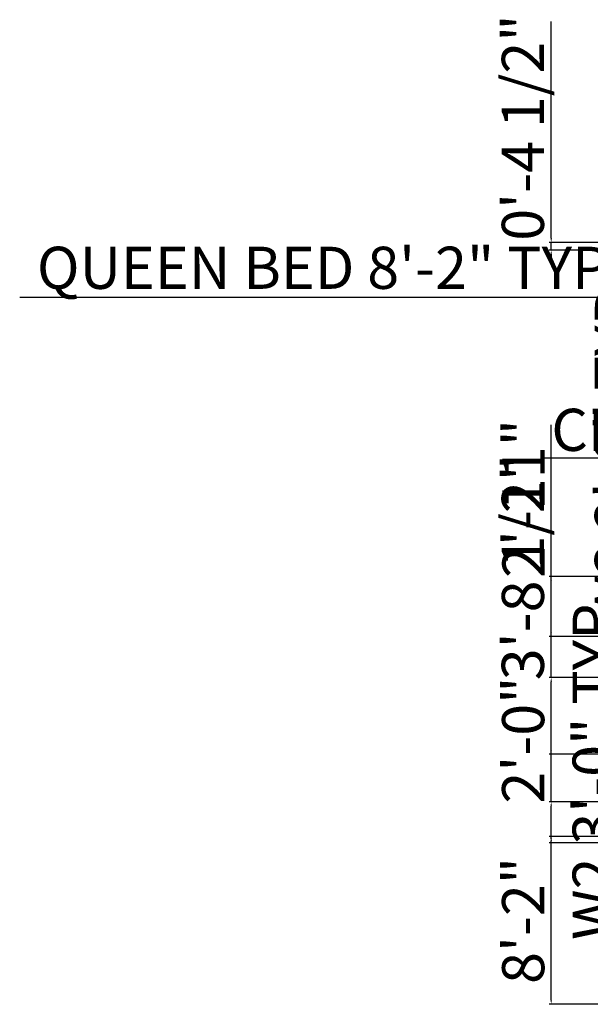
# Model space of a CAD drawing. Units: inches. Extents: x 1542 to 2523, y 1699 to 2449.
# Tile 1 of 7: x 1542 to 1875, y 1840 to 2414. Entities that reach past the tile are written whole.
import ezdxf

# ---------------------------------------------------------------- set-up
doc = ezdxf.new("R2010")
doc.units = ezdxf.units.IN
doc.layers.add('A-ANNO-DIMS', color=7, linetype='Continuous', lineweight=18)
doc.styles.get("Standard").update_dxf_attribs({"font": 'arial.ttf'})
doc.dimstyles.new('ISO-25', dxfattribs={"dimtxt": 24.5625, "dimasz": 2.5, "dimexe": 1.25, "dimexo": 0.625, "dimtad": 1, "dimlunit": 4, "dimtxsty": 'Standard', "dimcen": 2.5, "dimadec": 0, "dimazin": 0, "dimtfac": 10, "dimtmove": 0, "dimatfit": 3, "dimfxl": 1, "dimarcsym": 0})

# ---------------------------------------------------------------- blocks, each defined once
blk = doc.blocks.new('*D26')
at = {"layer": 'A-ANNO-DIMS', "color": 0, "lineweight": -2, "transparency": 16777216}
for p, q in [((2115.34, 2158.69), (1845.86, 2158.69)), ((2115.34, 2157.33), (2115.34, 2159.94)), ((2126.05, 2158.69), (2117.84, 2158.69)), ((2128.55, 2157.33), (2128.55, 2159.94))]:
    blk.add_line(p, q, dxfattribs=at)
at = {"layer": 'A-ANNO-DIMS', "color": 0, "transparency": 16777216}
for points in [[(2117.84, 2159.1), (2117.84, 2158.27), (2115.34, 2158.69)], [(2126.05, 2159.1), (2126.05, 2158.27), (2128.55, 2158.69)]]:
    blk.add_solid(points, dxfattribs=at)
at = {"layer": 'Defpoints', "color": 0, "transparency": 16777216}
for p in [(2115.34, 2158.69), (2115.34, 2156.7), (2128.55, 2156.7)]:
    blk.add_point(p, dxfattribs=at)
at = {"layer": 'A-ANNO-DIMS', "color": 0, "transparency": 16777216, "insert": (1979.35, 2172.01), "char_height": 24.5625, "attachment_point": 5}
blk.add_mtext('CHAIR 1\'-1" TYP.', dxfattribs=at)
blk = doc.blocks.new('*D28')
at = {"layer": 'A-ANNO-DIMS', "color": 0, "lineweight": -2, "transparency": 16777216}
for p, q in [((1905.99, 2054.87), (1905.99, 2270.35)), ((1903.01, 2054.87), (1907.24, 2054.87)), ((1905.99, 2033.33), (1905.99, 2052.37)), ((1903.01, 2030.83), (1907.24, 2030.83))]:
    blk.add_line(p, q, dxfattribs=at)
at = {"layer": 'A-ANNO-DIMS', "color": 0, "transparency": 16777216}
for points in [[(1905.57, 2052.37), (1906.4, 2052.37), (1905.99, 2054.87)], [(1905.57, 2033.33), (1906.4, 2033.33), (1905.99, 2030.83)]]:
    blk.add_solid(points, dxfattribs=at)
at = {"layer": 'Defpoints', "color": 0, "transparency": 16777216}
for p in [(1902.38, 2054.87), (1905.99, 2054.87), (1902.38, 2030.83)]:
    blk.add_point(p, dxfattribs=at)
at = {"layer": 'A-ANNO-DIMS', "color": 0, "transparency": 16777216, "insert": (1892.81, 2163.86), "char_height": 24.5625, "attachment_point": 5, "rotation": 90}
blk.add_mtext('W3 2\'-0" TYP.', dxfattribs=at)
blk = doc.blocks.new('*D32')
at = {"layer": 'A-ANNO-DIMS', "color": 0, "lineweight": -2, "transparency": 16777216}
for p, q in [((1922.46, 2274.54), (1926.04, 2274.54)), ((1924.79, 2272.04), (1924.79, 2257.33)), ((1922.46, 2254.83), (1926.04, 2254.83)), ((1924.79, 2254.83), (1924.79, 2060.84))]:
    blk.add_line(p, q, dxfattribs=at)
at = {"layer": 'A-ANNO-DIMS', "color": 0, "transparency": 16777216}
for points in [[(1924.37, 2272.04), (1925.21, 2272.04), (1924.79, 2274.54)], [(1924.37, 2257.33), (1925.21, 2257.33), (1924.79, 2254.83)]]:
    blk.add_solid(points, dxfattribs=at)
at = {"layer": 'Defpoints', "color": 0, "transparency": 16777216}
for p in [(1921.83, 2274.54), (1921.83, 2254.83), (1924.79, 2254.83)]:
    blk.add_point(p, dxfattribs=at)
at = {"layer": 'A-ANNO-DIMS', "color": 0, "transparency": 16777216, "insert": (1911.46, 2156.58), "char_height": 24.5625, "attachment_point": 5, "rotation": 90}
blk.add_mtext('WC 1\'-7 1/2"', dxfattribs=at)
blk = doc.blocks.new('*D36')
at = {"layer": 'A-ANNO-DIMS', "color": 0, "lineweight": -2, "transparency": 16777216}
for p, q in [((1897.82, 2125.68), (1891.79, 2125.68)), ((1893.04, 2123.18), (1893.04, 2092.15)), ((1897.82, 2089.65), (1891.79, 2089.65)), ((1893.04, 2089.65), (1893.04, 1874.17))]:
    blk.add_line(p, q, dxfattribs=at)
at = {"layer": 'A-ANNO-DIMS', "color": 0, "transparency": 16777216}
for points in [[(1892.62, 2123.18), (1893.46, 2123.18), (1893.04, 2125.68)], [(1892.62, 2092.15), (1893.46, 2092.15), (1893.04, 2089.65)]]:
    blk.add_solid(points, dxfattribs=at)
at = {"layer": 'Defpoints', "color": 0, "transparency": 16777216}
for p in [(1898.45, 2125.68), (1893.04, 2089.65), (1898.45, 2089.65)]:
    blk.add_point(p, dxfattribs=at)
at = {"layer": 'A-ANNO-DIMS', "color": 0, "transparency": 16777216, "insert": (1879.87, 1980.66), "char_height": 24.5625, "attachment_point": 5, "rotation": 90}
blk.add_mtext('W2 3\'-0" TYP.', dxfattribs=at)
blk = doc.blocks.new('*D38')
at = {"layer": 'A-ANNO-DIMS', "color": 0, "lineweight": -2, "transparency": 16777216}
for p, q in [((1907.17, 2252.37), (1542.11, 2252.37)), ((1907.17, 2238.32), (1907.17, 2253.62)), ((2002.53, 2252.37), (1909.67, 2252.37)), ((2005.03, 2238.32), (2005.03, 2253.62))]:
    blk.add_line(p, q, dxfattribs=at)
at = {"layer": 'A-ANNO-DIMS', "color": 0, "transparency": 16777216}
for points in [[(1909.67, 2252.79), (1909.67, 2251.95), (1907.17, 2252.37)], [(2002.53, 2252.79), (2002.53, 2251.95), (2005.03, 2252.37)]]:
    blk.add_solid(points, dxfattribs=at)
at = {"layer": 'Defpoints', "color": 0, "transparency": 16777216}
for p in [(1907.17, 2252.37), (1907.17, 2237.69), (2005.03, 2237.69)]:
    blk.add_point(p, dxfattribs=at)
at = {"layer": 'A-ANNO-DIMS', "color": 0, "transparency": 16777216, "insert": (1723.39, 2266.45), "char_height": 24.5625, "attachment_point": 5}
blk.add_mtext('QUEEN BED 8\'-2" TYP.', dxfattribs=at)
blk = doc.blocks.new('*D40')
at = {"layer": 'A-ANNO-DIMS', "color": 0, "lineweight": -2, "transparency": 16777216}
for p, q in [((1909.59, 1986.22), (1909.59, 2201.7)), ((1903.01, 1986.22), (1910.84, 1986.22)), ((1909.59, 1940.69), (1909.59, 1983.72)), ((1903.01, 1938.19), (1910.84, 1938.19))]:
    blk.add_line(p, q, dxfattribs=at)
at = {"layer": 'A-ANNO-DIMS', "color": 0, "transparency": 16777216}
for points in [[(1909.17, 1983.72), (1910, 1983.72), (1909.59, 1986.22)], [(1909.17, 1940.69), (1910, 1940.69), (1909.59, 1938.19)]]:
    blk.add_solid(points, dxfattribs=at)
at = {"layer": 'Defpoints', "color": 0, "transparency": 16777216}
for p in [(1902.38, 1986.22), (1909.59, 1986.22), (1902.38, 1938.19)]:
    blk.add_point(p, dxfattribs=at)
at = {"layer": 'A-ANNO-DIMS', "color": 0, "transparency": 16777216, "insert": (1896.42, 2095.21), "char_height": 24.5625, "attachment_point": 5, "rotation": 90}
blk.add_mtext('W1 4\'-0" TYP.', dxfattribs=at)
blk = doc.blocks.new('*D49')
at = {"layer": 'A-ANNO-DIMS', "color": 0, "lineweight": -2, "transparency": 16777216}
for p, q in [((1851.93, 1958.44), (1851.93, 2027.9)), ((2157.76, 1958.44), (1850.68, 1958.44)), ((1851.93, 1936.94), (1851.93, 1955.94)), ((2157.76, 1934.44), (1850.68, 1934.44))]:
    blk.add_line(p, q, dxfattribs=at)
at = {"layer": 'A-ANNO-DIMS', "color": 0, "transparency": 16777216}
for points in [[(1851.52, 1955.94), (1852.35, 1955.94), (1851.93, 1958.44)], [(1851.52, 1936.94), (1852.35, 1936.94), (1851.93, 1934.44)]]:
    blk.add_solid(points, dxfattribs=at)
at = {"layer": 'Defpoints', "color": 0, "transparency": 16777216}
for p in [(1851.93, 1958.44), (2158.38, 1958.44), (2158.38, 1934.44)]:
    blk.add_point(p, dxfattribs=at)
at = {"layer": 'A-ANNO-DIMS', "color": 0, "transparency": 16777216, "insert": (1838.77, 1994.42), "char_height": 24.562, "attachment_point": 5, "rotation": 90}
blk.add_mtext('2\'-0"', dxfattribs=at)
blk = doc.blocks.new('*D55')
at = {"layer": 'A-ANNO-DIMS', "color": 0, "lineweight": -2, "transparency": 16777216}
for p, q in [((1897.82, 1938.19), (1850.68, 1938.19)), ((1851.93, 1842.94), (1851.93, 1935.69)), ((1897.76, 1840.44), (1850.68, 1840.44))]:
    blk.add_line(p, q, dxfattribs=at)
at = {"layer": 'A-ANNO-DIMS', "color": 0, "transparency": 16777216}
for points in [[(1851.52, 1935.69), (1852.35, 1935.69), (1851.93, 1938.19)], [(1851.52, 1842.94), (1852.35, 1842.94), (1851.93, 1840.44)]]:
    blk.add_solid(points, dxfattribs=at)
at = {"layer": 'Defpoints', "color": 0, "transparency": 16777216}
for p in [(1851.93, 1938.19), (1898.45, 1938.19), (1898.38, 1840.44)]:
    blk.add_point(p, dxfattribs=at)
at = {"layer": 'A-ANNO-DIMS', "color": 0, "transparency": 16777216, "insert": (1838.77, 1889.31), "char_height": 24.562, "attachment_point": 5, "rotation": 90}
blk.add_mtext('8\'-2"', dxfattribs=at)
blk = doc.blocks.new('*D56')
at = {"layer": 'A-ANNO-DIMS', "color": 0, "lineweight": -2, "transparency": 16777216}
for p, q in [((1851.93, 2030.83), (1851.93, 2157.09)), ((1897.82, 2030.83), (1850.68, 2030.83)), ((1851.93, 1988.72), (1851.93, 2028.33)), ((1897.82, 1986.22), (1850.68, 1986.22))]:
    blk.add_line(p, q, dxfattribs=at)
at = {"layer": 'A-ANNO-DIMS', "color": 0, "transparency": 16777216}
for points in [[(1851.52, 2028.33), (1852.35, 2028.33), (1851.93, 2030.83)], [(1851.52, 1988.72), (1852.35, 1988.72), (1851.93, 1986.22)]]:
    blk.add_solid(points, dxfattribs=at)
at = {"layer": 'Defpoints', "color": 0, "transparency": 16777216}
for p in [(1851.93, 2030.83), (1898.45, 2030.83), (1898.45, 1986.22)]:
    blk.add_point(p, dxfattribs=at)
at = {"layer": 'A-ANNO-DIMS', "color": 0, "transparency": 16777216, "insert": (1838.6, 2095.21), "char_height": 24.562, "attachment_point": 5, "rotation": 90}
blk.add_mtext('3\'-8 1/2"', dxfattribs=at)
blk = doc.blocks.new('*D57')
at = {"layer": 'A-ANNO-DIMS', "color": 0, "lineweight": -2, "transparency": 16777216}
for p, q in [((1851.93, 2089.65), (1851.93, 2178.19)), ((1897.82, 2089.65), (1850.68, 2089.65)), ((1851.93, 2057.37), (1851.93, 2087.15)), ((1897.82, 2054.87), (1850.68, 2054.87))]:
    blk.add_line(p, q, dxfattribs=at)
at = {"layer": 'A-ANNO-DIMS', "color": 0, "transparency": 16777216}
for points in [[(1851.52, 2087.15), (1852.35, 2087.15), (1851.93, 2089.65)], [(1851.52, 2057.37), (1852.35, 2057.37), (1851.93, 2054.87)]]:
    blk.add_solid(points, dxfattribs=at)
at = {"layer": 'Defpoints', "color": 0, "transparency": 16777216}
for p in [(1851.93, 2089.65), (1898.45, 2089.65), (1898.45, 2054.87)]:
    blk.add_point(p, dxfattribs=at)
at = {"layer": 'A-ANNO-DIMS', "color": 0, "transparency": 16777216, "insert": (1838.98, 2135.17), "char_height": 24.562, "attachment_point": 5, "rotation": 90}
blk.add_mtext('2\'-11"', dxfattribs=at)
blk = doc.blocks.new('*D66')
at = {"layer": 'A-ANNO-DIMS', "color": 0, "lineweight": -2, "transparency": 16777216}
for p, q in [((1851.93, 2286.94), (1851.93, 2413.22)), ((1901.76, 2284.44), (1850.68, 2284.44)), ((1851.93, 2279.86), (1851.93, 2284.44)), ((1901.76, 2279.86), (1850.68, 2279.86)), ((1851.93, 2277.36), (1851.93, 2274.86))]:
    blk.add_line(p, q, dxfattribs=at)
at = {"layer": 'A-ANNO-DIMS', "color": 0, "transparency": 16777216}
for points in [[(1851.52, 2286.94), (1852.35, 2286.94), (1851.93, 2284.44)], [(1851.52, 2277.36), (1852.35, 2277.36), (1851.93, 2279.86)]]:
    blk.add_solid(points, dxfattribs=at)
at = {"layer": 'Defpoints', "color": 0, "transparency": 16777216}
for p in [(1851.93, 2284.44), (1902.38, 2284.44), (1902.38, 2279.86)]:
    blk.add_point(p, dxfattribs=at)
at = {"layer": 'A-ANNO-DIMS', "color": 0, "transparency": 16777216, "insert": (1838.61, 2351.33), "char_height": 24.562, "attachment_point": 5, "rotation": 90}
blk.add_mtext('0\'-4 1/2"', dxfattribs=at)

msp = doc.modelspace()

# ---------------------------------------------------------------- dimensions: what is measured, and where the dimension line sits
at = {"layer": 'A-ANNO-DIMS'}
for base, p1, p2, picture, middle in [((1851.933, 2284.439), (1902.383, 2279.859), (1902.383, 2284.439), '*D66', (1838.607, 2351.328)), ((1851.933, 2089.649), (1898.446, 2054.866), (1898.446, 2089.649), '*D57', (1838.976, 2135.172)), ((1851.933, 2030.833), (1898.446, 1986.223), (1898.446, 2030.833), '*D56', (1838.599, 2095.214)), ((1851.933, 1958.439), (2158.383, 1934.439), (2158.383, 1958.439), '*D49', (1838.767, 1994.42)), ((1851.933, 1938.191), (1898.383, 1840.439), (1898.446, 1938.191), '*D55', (1838.767, 1889.315))]:
    dim = msp.add_linear_dim(base=base, p1=p1, p2=p2, angle=90, dimstyle='ISO-25', override={"dimdec": 1, "dimlfac": 1, "dimrnd": 0, "dimzin": 1, "dimdsep": 46, "dimlunit": 4, "dimfrac": 2}, dxfattribs=at)
    dim.commit()
    dim.dimension.update_dxf_attribs({"geometry": picture, "text_midpoint": middle})
for base, p1, p2, angle, text, picture, middle in [((1907.173, 2252.371), (2005.029, 2237.692), (1907.173, 2237.692), 180, 'QUEEN BED <> TYP.', '*D38', (1723.39, 2266.45)), ((1924.788, 2254.826), (1921.831, 2274.545), (1921.831, 2254.826), 270, 'WC <>', '*D32', (1911.463, 2156.584)), ((1905.987, 2054.866), (1902.383, 2030.833), (1902.383, 2054.866), 90, 'W3 <> TYP.', '*D28', (1892.813, 2163.856)), ((2115.34, 2158.686), (2128.547, 2156.705), (2115.34, 2156.705), 180, 'CHAIR <> TYP.', '*D26', (1979.35, 2172.011)), ((1909.587, 1986.223), (1902.383, 1938.191), (1902.383, 1986.223), 90, 'W1 <> TYP.', '*D40', (1896.422, 2095.213)), ((1893.041, 2089.649), (1898.446, 2125.681), (1898.446, 2089.649), 270, 'W2 <> TYP.', '*D36', (1879.867, 1980.659))]:
    dim = msp.add_linear_dim(base=base, p1=p1, p2=p2, angle=angle, text=text, dimstyle='ISO-25', override={"dimdec": 1, "dimlfac": 1, "dimrnd": 0, "dimzin": 1, "dimdsep": 46, "dimlunit": 4, "dimfrac": 2}, dxfattribs=at)
    dim.commit()
    dim.dimension.update_dxf_attribs({"geometry": picture, "text_midpoint": middle})

doc.saveas('drawing.dxf')
